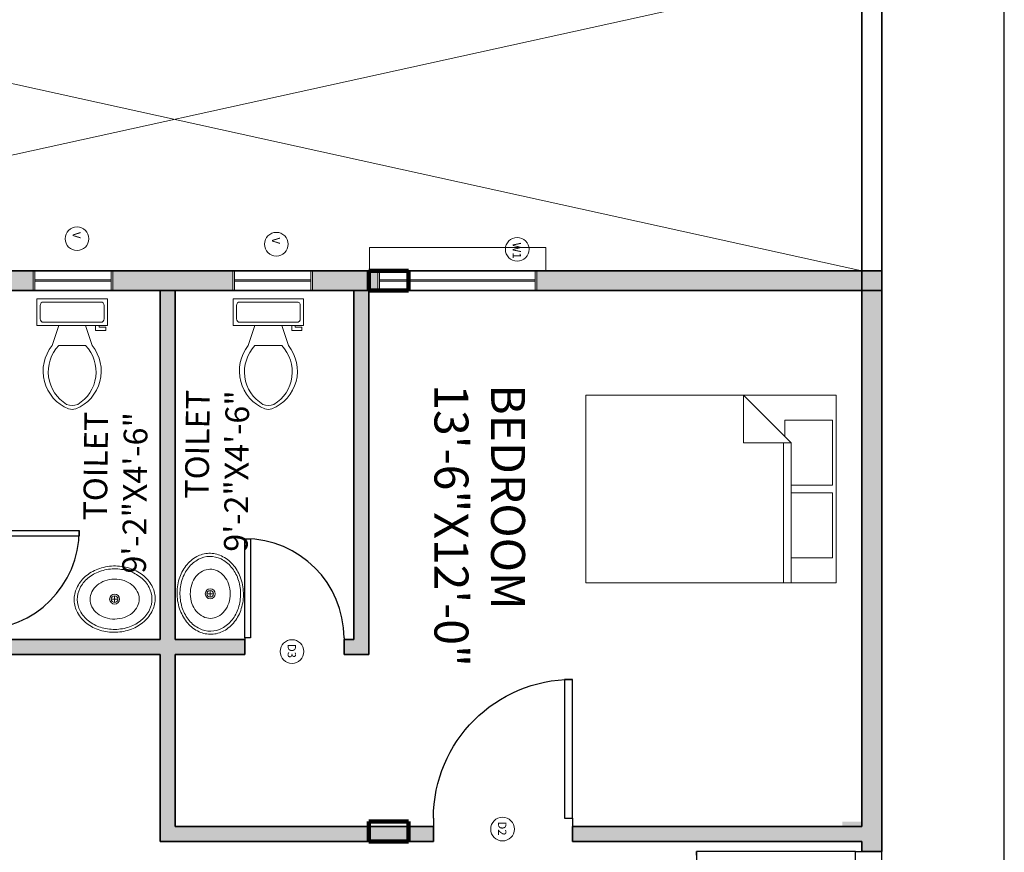
# Model space of a CAD drawing. Units: inches. Extents: x 7028582 to 7030319, y 63109697 to 63111305.
# Tile 9 of 18: x 7029402 to 7029699, y 63110278 to 63110530. Entities that reach past the tile are written whole.
import ezdxf

# ---------------------------------------------------------------- set-up
doc = ezdxf.new("R2010")
doc.units = ezdxf.units.IN
for name, color, linetype, lineweight in [('A-AREA-IDEN', 7, 'Continuous', 18), ('A-DOOR-IDEN', 20, 'Continuous', 13), ('A-FLOR-FIXT', 9, 'Continuous', 18), ('A-FLOR-OPEN', 7, 'Continuous', 13), ('A-GLAZ-IDEN', 20, 'Continuous', 13), ('A-WALL-PATT', 8, 'Continuous', 13), ('C-ANNO-DIMS', 7, 'Continuous', 18), ('doors', 20, 'Continuous', 25), ('furniture', 9, 'Continuous', 18), ('PILLARS', 220, 'Continuous', 100), ('S-COLS-PATT', 220, 'Continuous', 100), ('walls', 6, 'Continuous', 35), ('WINDOW SHADOW', 9, 'Continuous', 13), ('windows', 5, 'Continuous', 18)]:
    doc.layers.add(name, color=color, linetype=linetype, lineweight=lineweight)
doc.styles.get("Standard").update_dxf_attribs({"font": 'arial.ttf'})
doc.dimstyles.new('ISO-25', dxfattribs={"dimtxt": 2.5, "dimasz": 2.5, "dimexe": 1.25, "dimexo": 0.625, "dimtad": 1, "dimlunit": 4, "dimtxsty": 'Standard', "dimcen": 2.5, "dimadec": 0, "dimazin": 0, "dimtfac": 1, "dimtmove": 0, "dimatfit": 3, "dimfxl": 1, "dimarcsym": 0})

# ---------------------------------------------------------------- blocks, each defined once
blk = doc.blocks.new('*U2')
for p, q in [((0, 0), (0, -5)), ((30, 0), (30, -5))]:
    blk.add_line(p, q)
blk.add_lwpolyline([(0, 0), (0, 30), (1.75, 30), (1.75, 0)], close=True)
blk.add_arc((0, 0), 30, 0, 90)
blk = doc.blocks.new('Toilet - top')
for p, q in [((9.5, -6), (9.5, -2)), ((-10, -8.5), (-8, -8.5)), ((-10, -9.5), (-10, -8.5)), ((-8, -8.5), (-8, -8)), ((-7, -8), (-7, -9.5)), ((-4, -8), (-6, -14)), ((4, -8), (6, -14)), ((-7, -9.5), (-10, -9.5)), ((4, -14), (-4, -14))]:
    blk.add_line(p, q)
blk.add_lwpolyline([(10.5, -8), (10.5, 0), (-10.5, 0), (-10.5, -8)], close=True)
for points in [[(-9.5, -2), (-9.5, -6)], [(8.5, -1), (-8.5, -1)], [(-8.5, -7), (8.5, -7)]]:
    blk.add_lwpolyline(points)
for centre, radius, start, end in [((-8.62, -1.88), 0.884, 81.8699, 188.1301), ((8.62, -1.88), 0.884, 351.8699, 98.1301), ((-8.62, -6.12), 0.884, 171.8699, 278.1301), ((8.62, -6.12), 0.884, 261.8699, 8.1301), ((3.52, -21.58), 12.17, 141.4691, 247.9714), ((4.2, -21.82), 11.33, 136.3677, 238.9468), ((-3.52, -21.58), 12.17, 292.0284, 38.5307), ((-4.2, -21.82), 11.33, 301.053, 43.6321), ((0, -27.88), 4, 245.7318, 294.2682), ((0, -29), 4, 254.8605, 285.1395)]:
    blk.add_arc(centre, radius, start, end)
blk = doc.blocks.new('Sink - Oval top')
for p, q in [((-1, 0), (1, 0)), ((0, 1), (0, -1))]:
    blk.add_line(p, q)
for points in [[(-12.23, 0.39, 0.117634), (-11.46, -3.36, 0.104469), (-8.88, -6.8, 0.090016), (-5.08, -9.07, 0.08192), (-0.32, -10.02, 0.08192), (4.49, -9.38, 0.090016), (8.42, -7.36, 0.104469), (11.22, -4.09, 0.117634), (12.23, -0.39, 0.117634), (11.46, 3.36, 0.104469), (8.88, 6.8, 0.090016), (5.08, 9.07, 0.08192), (0.32, 10.02, 0.08192), (-4.49, 9.38, 0.090016), (-8.42, 7.36, 0.104469), (-11.22, 4.09, 0.117634)], [(-11.29, 0.16, 0.118622), (-10.52, -3.25, 0.104678), (-8.07, -6.36, 0.089562), (-4.54, -8.37, 0.081185), (-0.13, -9.15, 0.081185), (4.3, -8.49, 0.089562), (7.89, -6.58, 0.104678), (10.42, -3.55, 0.118622), (11.29, -0.16, 0.118622), (10.52, 3.25, 0.104678), (8.07, 6.36, 0.089562), (4.54, 8.37, 0.081185), (0.13, 9.15, 0.081185), (-4.3, 8.49, 0.089562), (-7.89, 6.58, 0.104678), (-10.42, 3.55, 0.118622)], [(-7.42, 0.08, 0.118283), (-6.91, -2.17, 0.104607), (-5.29, -4.21, 0.089718), (-2.97, -5.53, 0.081436), (-0.07, -6.04, 0.081436), (2.84, -5.59, 0.089718), (5.2, -4.33, 0.104607), (6.86, -2.32, 0.118283), (7.42, -0.08, 0.118283), (6.91, 2.17, 0.104607), (5.29, 4.21, 0.089718), (2.97, 5.53, 0.081436), (0.07, 6.04, 0.081436), (-2.84, 5.59, 0.089718), (-5.2, 4.33, 0.104607), (-6.86, 2.32, 0.118283)]]:
    blk.add_lwpolyline(points, format="xyb", close=True)
for radius in [1.5, 1]:
    blk.add_circle((0, 0), radius)
blk = doc.blocks.new('Bed - Queen')
for p, q in [((0, -80.00003), (0, 0)), ((0, 0), (59.99999, 0)), ((59.99999, 0), (59.99999, -80.00003)), ((7.99999, -1.2), (28.79998, -1.2)), ((7.99999, -14.4), (7.99999, -1.2)), ((28.79998, -1.2), (28.79998, -14.4)), ((31.19999, -1.2), (51.99999, -1.2)), ((31.19999, -14.4), (31.19999, -1.2)), ((51.99999, -1.2), (51.99999, -16.4)), ((0, -14.4), (44.8, -14.4)), ((59.99999, -29.6), (44.8, -14.4)), ((44.8, -14.4), (44.8, -29.6)), ((44.8, -16.8), (0, -16.8)), ((51.99999, -16.4), (46.79936, -16.4)), ((44.8, -29.6), (59.99999, -29.6)), ((59.99999, -80.00003), (0, -80.00003))]:
    blk.add_line(p, q)
blk = doc.blocks.new('WIN-SASH-24')
for p, q in [((24.05, 6), (0, 6)), ((0.5, 6), (0.5, 0)), ((23.55, 0), (23.55, 6)), ((23.55, 3.2), (0.5, 3.2)), ((0, 0), (24.05, 0)), ((23.55, 2.8), (0.5, 2.8))]:
    blk.add_line(p, q)
blk = doc.blocks.new('WIN-SASH-48')
for p, q in [((48.05, 6), (0, 6)), ((0.5, 6), (0.5, 0)), ((47.55, 0), (47.55, 6)), ((47.55, 3.2), (0.5, 3.2)), ((47.55, 2.8), (0.5, 2.8)), ((0, 0), (48.05, 0))]:
    blk.add_line(p, q)
blk = doc.blocks.new('WINDOW-SHADE-COURT-53')
for p, q in [((0, 0), (0, 7.06)), ((0, 7.06), (53.29, 7.06)), ((53.29, 7.06), (53.29, 0))]:
    blk.add_line(p, q)
blk = doc.blocks.new('COLUMN-RECT-PROFILE')
for p, q in [((11.91, 6), (0, 6)), ((0, 6), (0, 0)), ((11.91, 0), (11.91, 6)), ((0, 0), (11.91, 0))]:
    blk.add_line(p, q)
blk = doc.blocks.new('TAG-D2-ST-L')
blk.add_circle((3.58, 3.58), 3.58)
blk.add_text('D2', height=2.5, rotation=270).set_placement((2.23, 5.87))
blk = doc.blocks.new('TAG-D3-ST-L')
blk.add_circle((3.58, 3.58), 3.58)
blk.add_text('D3', height=2.5, rotation=270).set_placement((2.27, 5.87))
blk = doc.blocks.new('TAG-V-ST-L')
blk.add_circle((3.58, 3.58), 3.58)
blk.add_text('V', height=2.5, rotation=270).set_placement((2.23, 5.62))
blk = doc.blocks.new('TAG-W1-ST-L')
blk.add_circle((3.58, 3.58), 3.58)
blk.add_text('W1', height=2.5, rotation=270).set_placement((2.23, 5.64))
blk = doc.blocks.new('*D108')
at = {"layer": 'C-ANNO-DIMS', "color": 0, "lineweight": -2, "transparency": 16777216}
for p, q in [((7029662.21, 63110129.18), (7029662.21, 63111300.44)), ((7029664.71, 63111299.19), (7029696.71, 63111299.19)), ((7029699.21, 63110129.18), (7029699.21, 63111300.44))]:
    blk.add_line(p, q, dxfattribs=at)
at = {"layer": 'C-ANNO-DIMS', "color": 0, "lineweight": 100, "transparency": 16777216}
for points in [[(7029664.71, 63111299.61), (7029664.71, 63111298.77), (7029662.21, 63111299.19)], [(7029696.71, 63111299.61), (7029696.71, 63111298.77), (7029699.21, 63111299.19)]]:
    blk.add_solid(points, dxfattribs=at)
at = {"layer": 'Defpoints', "color": 0, "lineweight": 100, "transparency": 16777216}
for p in [(7029699.21, 63111299.19), (7029662.21, 63110128.56), (7029699.21, 63110128.56)]:
    blk.add_point(p, dxfattribs=at)
at = {"layer": 'C-ANNO-DIMS', "color": 0, "transparency": 16777216, "insert": (7029680.71, 63111301.09), "char_height": 2.5, "attachment_point": 5}
blk.add_mtext('3\'-1"', dxfattribs=at)

msp = doc.modelspace()

# ---------------------------------------------------------------- hatches: boundary and pattern name
at = {"layer": 'A-WALL-PATT'}
h = msp.add_hatch(color=256, dxfattribs=at)
h.dxf.hatch_style = 1
h.paths.add_polyline_path([(7029368.597, 63110454.057), (7029405.832, 63110454.057), (7029405.832, 63110448.057), (7029368.597, 63110448.057)])
h.paths.add_polyline_path([(7029384.705, 63110448.057), (7029389.205, 63110448.057), (7029389.205, 63110375.557), (7029384.705, 63110375.557)], flags=0)
h = msp.add_hatch(color=256, dxfattribs=at)
h.dxf.hatch_style = 1
h.paths.add_polyline_path([(7029429.881, 63110448.057), (7029466.152, 63110448.057), (7029466.152, 63110454.057), (7029429.881, 63110454.057)])
h = msp.add_hatch(color=256, dxfattribs=at)
h.dxf.hatch_style = 1
h.paths.add_polyline_path([(7029490.2, 63110448.057), (7029509.893, 63110448.057), (7029509.893, 63110454.057), (7029490.2, 63110454.057)])
h = msp.add_hatch(color=256, dxfattribs=at)
h.dxf.hatch_style = 1
h.paths.add_polyline_path([(7029557.941, 63110448.057), (7029662.205, 63110448.057), (7029662.205, 63110454.057), (7029585.16, 63110454.057), (7029557.941, 63110454.057)])
h = msp.add_hatch(color=256, dxfattribs=at)
h.dxf.hatch_style = 1
h.paths.add_polyline_path([(7029585.16, 63110454.057), (7029557.941, 63110454.057), (7029557.941, 63110448.057), (7029662.205, 63110448.057), (7029662.205, 63110454.057)])
h = msp.add_hatch(color=256, dxfattribs=at)
h.dxf.hatch_style = 1
h.paths.add_polyline_path([(7029384.705, 63110448.057), (7029389.205, 63110448.057), (7029389.205, 63110375.557), (7029384.705, 63110375.557)], flags=0)
h.paths.add_polyline_path([(7029384.705, 63110345.557), (7029389.205, 63110345.557), (7029389.205, 63110342.557), (7029444.205, 63110342.557), (7029444.205, 63110448.057), (7029448.705, 63110448.057), (7029448.705, 63110342.557), (7029469.705, 63110342.557), (7029469.705, 63110338.057), (7029448.705, 63110338.057), (7029448.705, 63110286.057), (7029526.726, 63110286.057), (7029526.726, 63110281.557), (7029444.205, 63110281.557), (7029444.205, 63110338.057), (7029389.205, 63110338.057), (7029389.205, 63110331.057), (7029384.705, 63110331.057)])
h = msp.add_hatch(color=256, dxfattribs=at)
h.dxf.hatch_style = 1
h.paths.add_polyline_path([(7029502.705, 63110448.057), (7029507.205, 63110448.057), (7029507.205, 63110338.057), (7029499.705, 63110338.057), (7029499.705, 63110342.557), (7029502.705, 63110342.557)], flags=17)
h = msp.add_hatch(color=256, dxfattribs=at)
h.dxf.hatch_style = 1
h.paths.add_polyline_path([(7029662.205, 63110448.057), (7029656.205, 63110448.057), (7029656.205, 63110286.057), (7029568.726, 63110286.057), (7029568.726, 63110281.557), (7029656.205, 63110281.557), (7029656.205, 63110278.557), (7029662.205, 63110278.557)])
at = {"layer": 'S-COLS-PATT'}
h = msp.add_hatch(color=256, dxfattribs=at)
h.dxf.hatch_style = 1
h.paths.add_polyline_path([(7029662.205, 63110454.057), (7029650.291, 63110454.057), (7029650.291, 63110448.057), (7029662.205, 63110448.057)])
h = msp.add_hatch(color=256, dxfattribs=at)
h.dxf.hatch_style = 1
h.paths.add_polyline_path([(7029662.205, 63110287.557), (7029650.291, 63110287.557), (7029650.291, 63110281.557), (7029662.205, 63110281.557)])

# ---------------------------------------------------------------- linework, layer by layer
at = {"layer": 'A-FLOR-OPEN'}
for p, q in [((7029656.205, 63110454.057), (7029240.705, 63110545.557)), ((7029240.705, 63110454.057), (7029656.205, 63110545.557))]:
    msp.add_line(p, q, dxfattribs=at)
at = {"layer": 'walls'}
for p, q in [((7029656.205, 63110545.557), (7029656.205, 63110448.057)), ((7029662.205, 63110542.557), (7029662.205, 63110457.057)), ((7029662.205, 63110454.057), (7029662.205, 63110457.057)), ((7029234.705, 63110454.057), (7029585.16, 63110454.057)), ((7029662.205, 63110454.057), (7029557.941, 63110454.057)), ((7029662.205, 63110454.057), (7029585.16, 63110454.057)), ((7029662.205, 63110454.057), (7029662.205, 63110448.057)), ((7029240.705, 63110448.057), (7029662.205, 63110448.057)), ((7029444.205, 63110342.557), (7029444.205, 63110448.057)), ((7029448.705, 63110342.557), (7029448.705, 63110448.057)), ((7029502.705, 63110342.557), (7029502.705, 63110448.057)), ((7029507.205, 63110338.057), (7029507.205, 63110448.057)), ((7029656.205, 63110286.057), (7029656.205, 63110448.057)), ((7029662.205, 63110278.557), (7029662.205, 63110448.057)), ((7029389.205, 63110342.557), (7029444.205, 63110342.557)), ((7029448.705, 63110342.557), (7029469.705, 63110342.557)), ((7029469.705, 63110338.057), (7029469.705, 63110342.557)), ((7029499.705, 63110342.557), (7029502.705, 63110342.557)), ((7029502.705, 63110342.557), (7029499.705, 63110342.557)), ((7029499.705, 63110342.557), (7029499.705, 63110338.057)), ((7029389.205, 63110338.057), (7029444.205, 63110338.057)), ((7029444.205, 63110281.557), (7029444.205, 63110338.057)), ((7029448.705, 63110286.057), (7029448.705, 63110338.057)), ((7029448.705, 63110338.057), (7029469.705, 63110338.057)), ((7029499.705, 63110338.057), (7029507.205, 63110338.057)), ((7029448.705, 63110286.057), (7029526.726, 63110286.057)), ((7029526.726, 63110281.557), (7029526.726, 63110286.057)), ((7029568.726, 63110286.057), (7029656.205, 63110286.057)), ((7029568.726, 63110286.057), (7029568.726, 63110281.557)), ((7029444.205, 63110281.557), (7029526.726, 63110281.557)), ((7029568.726, 63110281.557), (7029656.205, 63110281.557)), ((7029656.205, 63110278.557), (7029656.205, 63110281.557)), ((7029656.205, 63110281.557), (7029656.205, 63110278.557)), ((7029656.205, 63110278.557), (7029662.205, 63110278.557))]:
    msp.add_line(p, q, dxfattribs=at)
at = {"layer": 'windows'}
for p, q in [((7029405.832, 63110448.057), (7029405.832, 63110454.057)), ((7029429.881, 63110454.057), (7029429.881, 63110448.057)), ((7029466.152, 63110448.057), (7029466.152, 63110454.057)), ((7029490.2, 63110454.057), (7029490.2, 63110448.057)), ((7029509.893, 63110448.057), (7029509.893, 63110454.057)), ((7029557.941, 63110454.057), (7029557.941, 63110448.057))]:
    msp.add_line(p, q, dxfattribs=at)

# ---------------------------------------------------------------- block references
at = {"layer": 'A-DOOR-IDEN'}
for name, p in [('TAG-D3-ST-L', (7029480.418, 63110335.381)), ('TAG-D2-ST-L', (7029544.022, 63110281.722))]:
    msp.add_blockref(name, p, dxfattribs=at)
at = {"layer": 'A-FLOR-FIXT', "xscale": -1.013555723357934, "yscale": 1.013555723357934, "zscale": 1.013555723357934}
for p in [(7029417.569, 63110445.605), (7029476.859, 63110445.605)]:
    msp.add_blockref('Toilet - top', p, dxfattribs=at)
at = {"layer": 'A-FLOR-FIXT', "xscale": -1, "rotation": 270}
msp.add_blockref('Sink - Oval top', (7029459.289, 63110356.416), dxfattribs=at)
at = {"layer": 'A-FLOR-FIXT', "xscale": -1}
msp.add_blockref('Sink - Oval top', (7029430.396, 63110354.801), dxfattribs=at)
at = {"layer": 'A-GLAZ-IDEN'}
for name, p in [('TAG-V-ST-L', (7029415.449, 63110460.151)), ('TAG-V-ST-L', (7029475.673, 63110458.489)), ('TAG-W1-ST-L', (7029548.45, 63110456.953))]:
    msp.add_blockref(name, p, dxfattribs=at)
at = {"layer": 'doors', "rotation": 270}
msp.add_blockref('*U2', (7029389.705, 63110375.557), dxfattribs=at)
at = {"layer": 'doors'}
msp.add_blockref('*U2', (7029469.705, 63110343.057), dxfattribs=at)
at = {"layer": 'doors', "xscale": -1.399999999999999, "yscale": 1.399999999999999, "zscale": 1.399999999999999}
msp.add_blockref('*U2', (7029568.726, 63110288.557), dxfattribs=at)
at = {"layer": 'doors', "xscale": -1.599999999999999, "yscale": 1.599999999999999, "zscale": 1.599999999999999, "rotation": 90}
msp.add_blockref('*U2', (7029654.205, 63110278.557), dxfattribs=at)
at = {"layer": 'furniture', "xscale": -0.9464141645025947, "yscale": 0.9464141645025947, "zscale": 0.9464141645025947, "rotation": 270}
msp.add_blockref('Bed - Queen', (7029648.437, 63110359.688), dxfattribs=at)
at = {"layer": 'PILLARS'}
for p in [(7029507.238, 63110448.057), (7029507.238, 63110281.557)]:
    msp.add_blockref('COLUMN-RECT-PROFILE', p, dxfattribs=at)
at = {"layer": 'WINDOW SHADOW'}
msp.add_blockref('WINDOW-SHADE-COURT-53', (7029507.356, 63110454.057), dxfattribs=at)
at = {"layer": 'windows'}
for name, p in [('WIN-SASH-24', (7029405.832, 63110448.057)), ('WIN-SASH-24', (7029466.152, 63110448.057)), ('WIN-SASH-48', (7029509.893, 63110448.057))]:
    msp.add_blockref(name, p, dxfattribs=at)

# ---------------------------------------------------------------- texts
at = {"layer": 'A-AREA-IDEN'}
for s, width, gutter_width, insert, char_height, attachment_point, rotation in [('TOILET\\P9\'-2"X4\'-6"', 42.97461, 35.821, (7029452.002, 63110418.065), 7.16426, 3, 89.3536), ('BEDROOM\\P13\'-6"X12\'-0"', 82.04322, 51.315, (7029527.033, 63110419.737), 10.26307, 7, 270), ('TOILET\\P9\'-2"X4\'-6"', 42.97461, 35.821, (7029421.278, 63110411.477), 7.16426, 3, 89.3536)]:
    msp.add_mtext_dynamic_manual_height_columns(s, width=width, gutter_width=gutter_width, heights=[0], dxfattribs=dict(at, insert=insert, char_height=char_height, attachment_point=attachment_point, rotation=rotation))

# ---------------------------------------------------------------- dimensions: what is measured, and where the dimension line sits
at = {"layer": 'C-ANNO-DIMS'}
dim = msp.add_linear_dim(base=(7029699.205, 63111299.19), p1=(7029662.205, 63110128.557), p2=(7029699.205, 63110128.557), dimstyle='ISO-25', override={"dimdec": 1, "dimlfac": 1, "dimrnd": 0, "dimzin": 1, "dimdsep": 46, "dimlunit": 4, "dimfrac": 2}, dxfattribs=at)
dim.commit()
dim.dimension.update_dxf_attribs({"geometry": '*D108', "text_midpoint": (7029680.705, 63111301.092)})

doc.saveas('drawing.dxf')
